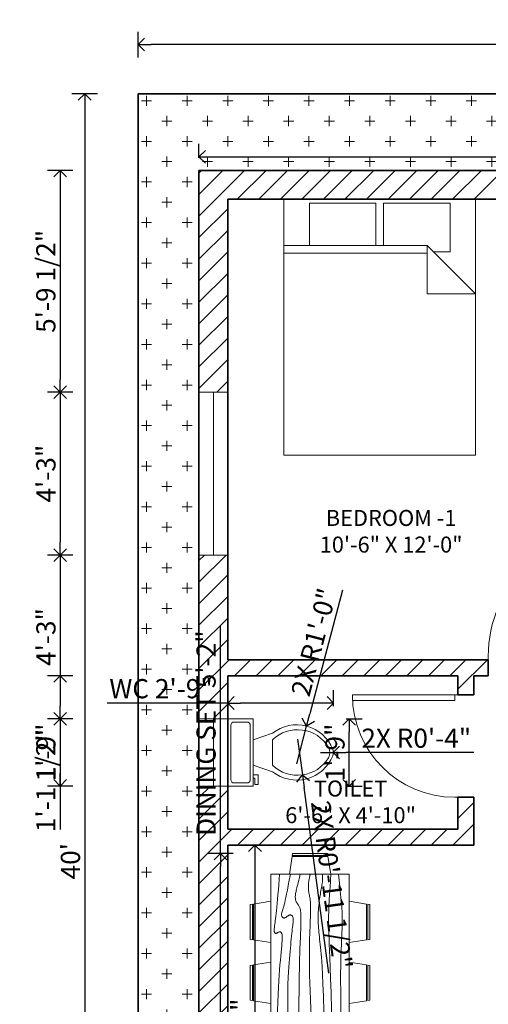
# Model space of a CAD drawing. Units: inches. Extents: x 686 to 1065, y 83 to 664.
# Tile 3 of 5: x 686 to 833, y 308 to 616. Entities that reach past the tile are written whole.
import ezdxf

# ---------------------------------------------------------------- set-up
doc = ezdxf.new("R2010")
doc.units = ezdxf.units.IN
for name, color, linetype, lineweight in [('A-ANNO-DIMS', 2, 'Continuous', 18), ('A-AREA-IDEN', 7, 'Continuous', 20), ('A-DOOR', 4, 'Continuous', 20), ('A-FLOR-FIXT', 9, 'Continuous', 18), ('A-FURN', 8, 'Continuous', 18), ('A-GLAZ', 172, 'Continuous', 18), ('A-WALL', 7, 'Continuous', 35), ('A-WALL-PATT', 253, 'Continuous', 13), ('C-PROP', 7, 'Continuous', 35), ('L-SITE-PATT', 94, 'Continuous', 13)]:
    doc.layers.add(name, color=color, linetype=linetype, lineweight=lineweight)
doc.styles.get("Standard").update_dxf_attribs({"font": 'arial.ttf'})
doc.dimstyles.new('ISO-25', dxfattribs={"dimtxt": 6, "dimasz": 4, "dimexe": 4, "dimexo": 4, "dimtad": 1, "dimdec": 1, "dimlunit": 3, "dimtxsty": 'Standard', "dimblk": 'OPEN90', "dimcen": 2.5, "dimadec": 0, "dimazin": 0, "dimtfac": 1, "dimtdec": 1, "dimtmove": 0, "dimatfit": 3, "dimfxl": 4, "dimfxlon": 1, "dimarcsym": 0})

# ---------------------------------------------------------------- blocks, each defined once
blk = doc.blocks.new('_Open90')
at = {"color": 0, "linetype": 'ByBlock', "lineweight": -2}
for p, q in [((0, 0), (-1, 0)), ((-0.5, 0.5), (0, 0)), ((0, 0), (-0.5, -0.5))]:
    blk.add_line(p, q, dxfattribs=at)
blk = doc.blocks.new('*D11')
at = {"layer": 'A-ANNO-DIMS', "color": 0, "lineweight": -2, "transparency": 16777216}
for p, q in [((742.37, 572.73), (742.37, 577.04)), ((1011.37, 572.73), (1011.37, 577.04)), ((746.37, 573.04), (1007.37, 573.04))]:
    blk.add_line(p, q, dxfattribs=at)
at = {"layer": 'Defpoints', "color": 0, "transparency": 16777216}
for p in [(1011.37, 573.04), (742.37, 568.73), (1011.37, 568.73)]:
    blk.add_point(p, dxfattribs=at)
at = {"layer": 'A-ANNO-DIMS', "color": 0, "lineweight": -2, "transparency": 16777216, "xscale": 4, "yscale": 4, "zscale": 4, "rotation": 180}
blk.add_blockref('_Open90', (742.37, 573.04), dxfattribs=at)
at = {"layer": 'A-ANNO-DIMS', "color": 0, "lineweight": -2, "transparency": 16777216, "xscale": 4, "yscale": 4, "zscale": 4}
blk.add_blockref('_Open90', (1011.37, 573.04), dxfattribs=at)
at = {"layer": 'A-ANNO-DIMS', "color": 0, "transparency": 16777216, "insert": (876.87, 576.73), "char_height": 6, "attachment_point": 5}
blk.add_mtext('22\'-5"', dxfattribs=at)
blk = doc.blocks.new('*D13')
at = {"layer": 'A-ANNO-DIMS', "color": 0, "lineweight": -2, "transparency": 16777216}
for p, q in [((755.89, 357.73), (763.89, 357.73)), ((759.89, 353.73), (759.89, 247.73)), ((755.89, 243.73), (763.89, 243.73))]:
    blk.add_line(p, q, dxfattribs=at)
at = {"layer": 'Defpoints', "color": 0, "transparency": 16777216}
for p in [(751.37, 357.73), (751.37, 243.73), (759.89, 243.73)]:
    blk.add_point(p, dxfattribs=at)
at = {"layer": 'A-ANNO-DIMS', "color": 0, "lineweight": -2, "transparency": 16777216, "xscale": 4, "yscale": 4, "zscale": 4}
for p, rotation in [((759.89, 357.73), 90), ((759.89, 243.73), 270)]:
    blk.add_blockref('_Open90', p, dxfattribs=dict(at, rotation=rotation))
at = {"layer": 'A-ANNO-DIMS', "color": 0, "transparency": 16777216, "insert": (756.2, 300.73), "char_height": 6, "attachment_point": 5, "rotation": 90}
blk.add_mtext('8\'-1"', dxfattribs=at)
blk = doc.blocks.new('Toilet - top')
for p, q in [((9.5, -6), (9.5, -2)), ((-10, -8.5), (-8, -8.5)), ((-10, -9.5), (-10, -8.5)), ((-8, -8.5), (-8, -8)), ((-7, -8), (-7, -9.5)), ((-4, -8), (-6, -14)), ((4, -8), (6, -14)), ((-7, -9.5), (-10, -9.5)), ((4, -14), (-4, -14))]:
    blk.add_line(p, q)
blk.add_lwpolyline([(10.5, -8), (10.5, 0), (-10.5, 0), (-10.5, -8)], close=True)
for points in [[(-9.5, -2), (-9.5, -6)], [(8.5, -1), (-8.5, -1)], [(-8.5, -7), (8.5, -7)]]:
    blk.add_lwpolyline(points)
for centre, radius, start, end in [((-8.62, -1.88), 0.884, 81.8699, 188.1301), ((8.62, -1.88), 0.884, 351.8699, 98.1301), ((-8.62, -6.12), 0.884, 171.8699, 278.1301), ((8.62, -6.12), 0.884, 261.8699, 8.1301), ((3.52, -21.58), 12.17, 141.4691, 247.9714), ((4.2, -21.82), 11.33, 136.3677, 238.9468), ((-3.52, -21.58), 12.17, 292.0284, 38.5307), ((-4.2, -21.82), 11.33, 301.053, 43.6321), ((0, -27.88), 4, 245.7318, 294.2682), ((0, -29), 4, 254.8605, 285.1395)]:
    blk.add_arc(centre, radius, start, end)
blk = doc.blocks.new('Bed - Queen')
for p, q in [((0, -80.00003), (0, 0)), ((0, 0), (59.99999, 0)), ((59.99999, 0), (59.99999, -80.00003)), ((7.99999, -1.2), (28.79998, -1.2)), ((7.99999, -14.4), (7.99999, -1.2)), ((28.79998, -1.2), (28.79998, -14.4)), ((31.19999, -1.2), (51.99999, -1.2)), ((31.19999, -14.4), (31.19999, -1.2)), ((51.99999, -1.2), (51.99999, -16.4)), ((0, -14.4), (44.8, -14.4)), ((59.99999, -29.6), (44.8, -14.4)), ((44.8, -14.4), (44.8, -29.6)), ((44.8, -16.8), (0, -16.8)), ((51.99999, -16.4), (46.79936, -16.4)), ((44.8, -29.6), (59.99999, -29.6)), ((59.99999, -80.00003), (0, -80.00003))]:
    blk.add_line(p, q)
blk = doc.blocks.new('Dining Set - 36 x 72 in.')
for p, q in [((-22, 27.5), (-22.1562, 26.50042)), ((-22, 27.5), (-6, 27.5)), ((-5.8437, 26.49966), (-6, 27.5)), ((6, 27.5), (5.8438, 26.50042)), ((6, 27.5), (22, 27.5)), ((22.1563, 26.49966), (22, 27.5)), ((-22.2343, 26.00059), (-23.4847, 17.99762)), ((-22.2304, 26), (-5.7608, 26)), ((-5.8416, 26.5), (-22.1534, 26.5)), ((-4.5152, 17.99762), (-5.7655, 25.99926)), ((5.7657, 26.00059), (4.5153, 17.99762)), ((5.7696, 26), (22.2392, 26)), ((22.1584, 26.5), (5.8466, 26.5)), ((23.4848, 17.99762), (22.2345, 25.99926)), ((36, 18), (-36, 18)), ((-36, 18), (-36, -18)), ((36, -18), (36, 18)), ((-44.0006, 8.23428), (-35.9976, 9.48474)), ((44.0006, 8.23428), (35.9976, 9.48474)), ((-45.5, 8), (-44.5004, 8.15617)), ((-45.5, 8), (-45.5, -8)), ((-44.5, -8.15843), (-44.5, 8.15338)), ((-44, 8.23041), (-44, -8.23915)), ((44, 8.23041), (44, -8.23915)), ((44.5, -8.15843), (44.5, 8.15338)), ((45.5, 8), (44.5005, 8.15617)), ((45.5, 8), (45.5, -8)), ((-44.4997, -8.15631), (-45.5, -8)), ((-35.9976, -9.48476), (-43.9993, -8.2345)), ((35.9976, -9.48476), (43.9993, -8.2345)), ((44.4997, -8.15631), (45.5, -8)), ((-36, -18), (36, -18)), ((-22.2343, -26.0006), (-23.4847, -17.99762)), ((-4.5152, -17.99762), (-5.7655, -25.99928)), ((5.7657, -26.0006), (4.5153, -17.99762)), ((23.4848, -17.99762), (22.2345, -25.99928)), ((-22.2304, -26), (-5.7608, -26)), ((-22, -27.5), (-22.1562, -26.50044)), ((-5.8416, -26.5), (-22.1534, -26.5)), ((-5.8437, -26.49967), (-6, -27.5)), ((5.7696, -26), (22.2392, -26)), ((6, -27.5), (5.8438, -26.50044)), ((22.1584, -26.5), (5.8466, -26.5)), ((22.1563, -26.49967), (22, -27.5)), ((-22, -27.5), (-6, -27.5)), ((6, -27.5), (22, -27.5))]:
    blk.add_line(p, q)
for points in [[(-36, 15), (-31.1772, 14.97754), (-26.8079, 14.91406), (-22.8538, 14.81543), (-19.276, 14.6875), (-16.0362, 14.53613), (-13.0957, 14.36718), (-10.4159, 14.18652), (-7.9583, 14), (-5.6904, 13.81315), (-3.6035, 13.63021), (-1.6954, 13.45508), (0.0365, 13.29166), (1.5945, 13.14388), (2.9811, 13.01562), (4.1988, 12.9108), (5.25, 12.83333), (6.1393, 12.78613), (6.8802, 12.76823), (7.4883, 12.77767), (7.9792, 12.8125), (8.3685, 12.87077), (8.6719, 12.95052), (8.9049, 13.0498), (9.0833, 13.16666), (9.2205, 13.29899), (9.3216, 13.44401), (9.3895, 13.59879), (9.4271, 13.76041), (9.4373, 13.92594), (9.4232, 14.09245), (9.3875, 14.257), (9.3333, 14.41666), (9.2638, 14.56917), (9.1836, 14.71484), (9.0975, 14.85465), (9.0104, 14.98958), (8.9272, 15.1206), (8.8529, 15.2487), (8.7922, 15.37483), (8.75, 15.5), (8.7305, 15.62467), (8.7344, 15.74739), (8.7617, 15.86621), (8.8125, 15.97916), (8.8867, 16.08431), (8.9844, 16.17968), (9.1055, 16.26334), (9.25, 16.33333), (9.4189, 16.38802), (9.6172, 16.42708), (9.8506, 16.45052), (10.125, 16.45833), (10.4463, 16.45052), (10.8203, 16.42708), (11.2529, 16.38802), (11.75, 16.33333), (12.3184, 16.26318), (12.9694, 16.17838), (13.7151, 16.07991), (14.5677, 15.96875), (15.5395, 15.84586), (16.6426, 15.71224), (17.8893, 15.56884), (19.2917, 15.41666), (20.859, 15.25667), (22.5879, 15.08984), (24.4721, 14.91715), (26.5052, 14.73958), (28.6809, 14.5581), (30.9929, 14.3737), (33.4347, 14.18733), (36, 14)], [(-36, 10), (-28.9766, 10.14274), (-23.1725, 10.20442), (-18.4241, 10.19775), (-14.5677, 10.13541), (-11.4399, 10.03011), (-8.877, 9.89453), (-6.7154, 9.74137), (-4.7917, 9.58333), (-2.9698, 9.43082), (-1.2246, 9.28515), (0.4415, 9.14534), (2.026, 9.01041), (3.5266, 8.87939), (4.9408, 8.7513), (6.266, 8.62516), (7.5, 8.5), (8.6411, 8.37549), (9.6914, 8.2539), (10.6538, 8.13818), (11.5312, 8.03125), (12.3267, 7.93603), (13.043, 7.85547), (13.6831, 7.79248), (14.25, 7.75), (14.7471, 7.7303), (15.1797, 7.73307), (15.5537, 7.75732), (15.875, 7.80208), (16.1494, 7.86637), (16.3828, 7.94922), (16.5811, 8.04964), (16.75, 8.16666), (16.8944, 8.29915), (17.0143, 8.44531), (17.1089, 8.60319), (17.1771, 8.77083), (17.218, 8.94629), (17.2305, 9.1276), (17.2137, 9.31282), (17.1667, 9.5), (17.0895, 9.6875), (16.987, 9.875), (16.8649, 10.0625), (16.7292, 10.25), (16.5856, 10.4375), (16.4401, 10.625), (16.2985, 10.8125), (16.1667, 11), (16.05, 11.18733), (15.9518, 11.3737), (15.8752, 11.5581), (15.8229, 11.73958), (15.798, 11.91715), (15.8034, 12.08984), (15.842, 12.25667), (15.9167, 12.41666), (16.0295, 12.56836), (16.1784, 12.70833), (16.3605, 12.83268), (16.5729, 12.9375), (16.8127, 13.01888), (17.0768, 13.07291), (17.3625, 13.0957), (17.6667, 13.08333), (17.9894, 13.03312), (18.3418, 12.94726), (18.7382, 12.82918), (19.1927, 12.68229), (19.7195, 12.51001), (20.3327, 12.31575), (21.0465, 12.10294), (21.875, 11.875), (22.8357, 11.63354), (23.959, 11.37304), (25.2786, 11.08618), (26.8282, 10.76562), (28.6414, 10.40405), (30.752, 9.99414), (33.1936, 9.52856), (36, 9)], [(-36, 5.5), (-30.7157, 5.3348), (-26.069, 5.20963), (-21.9946, 5.11767), (-18.4271, 5.05208), (-15.3009, 5.00602), (-12.5508, 4.97265), (-10.1112, 4.94515), (-7.9167, 4.91666), (-5.909, 4.88167), (-4.0586, 4.83984), (-2.3429, 4.79215), (-0.7396, 4.73958), (0.7739, 4.6831), (2.22, 4.6237), (3.6213, 4.56233), (5, 4.5), (6.373, 4.43782), (7.7344, 4.3776), (9.0723, 4.32129), (10.375, 4.27083), (11.6309, 4.22819), (12.8281, 4.19531), (13.9551, 4.17415), (15, 4.16666), (15.954, 4.17448), (16.819, 4.19791), (17.6001, 4.23698), (18.3021, 4.29166), (18.9299, 4.36198), (19.4883, 4.44791), (19.9823, 4.54948), (20.4167, 4.66666), (20.7969, 4.79899), (21.1302, 4.94401), (21.4245, 5.09879), (21.6875, 5.26041), (21.9271, 5.42594), (22.1511, 5.59245), (22.3672, 5.757), (22.5834, 5.91666), (22.8065, 6.06868), (23.0404, 6.21093), (23.2879, 6.34147), (23.5521, 6.45833), (23.8358, 6.55957), (24.142, 6.64323), (24.4735, 6.70735), (24.8334, 6.75), (25.2235, 6.76969), (25.642, 6.76692), (26.0858, 6.74267), (26.5521, 6.69791), (27.0379, 6.63362), (27.5404, 6.55078), (28.0565, 6.45036), (28.5834, 6.33333), (29.1242, 6.19987), (29.7071, 6.04687), (30.3661, 5.87044), (31.1354, 5.66666), (32.0493, 5.43164), (33.142, 5.16146), (34.4475, 4.85221), (36, 4.5)], [(-36, -1), (-30.7915, -0.6591), (-26.0195, -0.38216), (-21.6519, -0.16284), (-17.6563, 0.00521), (-14.0005, 0.12833), (-10.6523, 0.21289), (-7.5796, 0.26522), (-4.75, 0.29166), (-2.134, 0.29793), (0.2878, 0.28711), (2.5317, 0.26163), (4.6146, 0.22396), (6.5529, 0.17651), (8.3633, 0.12174), (10.0623, 0.06209), (11.6667, 0), (13.1899, -0.06201), (14.6341, -0.1211), (15.9982, -0.17432), (17.2813, -0.21875), (18.4823, -0.25147), (19.6003, -0.26953), (20.6343, -0.27002), (21.5834, -0.25), (22.4481, -0.20768), (23.2357, -0.14584), (23.9549, -0.06836), (24.6146, 0.02083), (25.2235, 0.11784), (25.7904, 0.21875), (26.3241, 0.31966), (26.8334, 0.41666), (27.3265, 0.50618), (27.8099, 0.58593), (28.2894, 0.65397), (28.7709, 0.70833), (29.2601, 0.74707), (29.763, 0.76823), (30.2855, 0.76985), (30.8334, 0.75), (31.4088, 0.70784), (31.9994, 0.64713), (32.589, 0.57275), (33.1615, 0.48958), (33.7008, 0.4025), (34.1908, 0.3164), (34.6153, 0.23616), (34.9584, 0.16666), (35.2099, 0.11165), (35.3848, 0.07031), (35.504, 0.04069), (35.5886, 0.02083), (35.6594, 0.00879), (35.7377, 0.0026), (35.8442, 0.00032), (36, 0)], [(-36, -6.5), (-27.1843, -6.31267), (-20.084, -6.1263), (-14.469, -5.9419), (-10.1094, -5.76042), (-6.7752, -5.58285), (-4.2363, -5.41016), (-2.2629, -5.24333), (-0.625, -5.08334), (0.8708, -4.93099), (2.2715, -4.78646), (3.5872, -4.64974), (4.8281, -4.52084), (6.0046, -4.39974), (7.127, -4.28646), (8.2053, -4.18099), (9.25, -4.08334), (10.2705, -3.99382), (11.2734, -3.91407), (12.2647, -3.84603), (13.25, -3.79167), (14.2354, -3.75293), (15.2266, -3.73177), (16.2295, -3.73015), (17.25, -3.75), (18.2912, -3.79248), (19.3451, -3.85547), (20.4009, -3.93604), (21.4479, -4.03125), (22.4754, -4.13819), (23.4727, -4.25391), (24.4289, -4.37549), (25.3334, -4.5), (26.1785, -4.62492), (26.9694, -4.74935), (27.7145, -4.87281), (28.4219, -4.99479), (29.1, -5.11483), (29.7572, -5.23242), (30.4016, -5.34709), (31.0417, -5.45834), (31.6837, -5.56437), (32.3262, -5.65821), (32.9658, -5.73153), (33.599, -5.77604), (34.2224, -5.78345), (34.8327, -5.74545), (35.4264, -5.65373), (36, -5.5)], [(-36, -10), (-26.4022, -9.81299), (-18.4675, -9.62891), (-11.9839, -9.45069), (-6.7396, -9.28125), (-2.5226, -9.12354), (0.8789, -8.98047), (3.6769, -8.85498), (6.0833, -8.75), (8.2767, -8.66765), (10.3021, -8.60677), (12.1712, -8.56543), (13.8958, -8.54167), (15.4876, -8.53353), (16.9583, -8.53907), (18.3197, -8.55632), (19.5834, -8.58334), (20.7616, -8.61841), (21.8685, -8.66081), (22.9188, -8.71004), (23.9271, -8.76563), (24.9081, -8.82707), (25.8763, -8.89388), (26.8465, -8.96558), (27.8334, -9.04167), (28.8474, -9.12118), (29.8828, -9.20117), (30.93, -9.27824), (31.9792, -9.34896), (33.0205, -9.40991), (34.0443, -9.45768), (35.0407, -9.48885), (36, -9.5)], [(-36, -14.5), (-30.0881, -14.33513), (-25.0332, -14.21224), (-20.7312, -14.12647), (-17.0781, -14.07292), (-13.97, -14.04671), (-11.3027, -14.04297), (-8.9724, -14.05681), (-6.875, -14.08334), (-4.9224, -14.11833), (-3.0905, -14.16016), (-1.3709, -14.20785), (0.2448, -14.26042), (1.7647, -14.3169), (3.1973, -14.3763), (4.5507, -14.43767), (5.8333, -14.5), (7.0554, -14.5621), (8.235, -14.62175), (9.3922, -14.67652), (10.5469, -14.72396), (11.7192, -14.76164), (12.929, -14.78711), (14.1965, -14.79794), (15.5417, -14.79167), (16.9933, -14.76424), (18.6152, -14.70508), (20.4804, -14.60197), (22.6615, -14.44271), (25.2312, -14.21509), (28.2624, -13.9069), (31.8277, -13.50594), (36, -13)]]:
    blk.add_lwpolyline(points)
blk = doc.blocks.new('*D17')
at = {"layer": 'A-ANNO-DIMS', "color": 0, "lineweight": -2, "transparency": 16777216}
for p, q in [((723.37, 604.13), (723.37, 612.13)), ((1023.37, 604.13), (1023.37, 612.13)), ((1019.37, 608.13), (727.37, 608.13))]:
    blk.add_line(p, q, dxfattribs=at)
at = {"layer": 'Defpoints', "color": 0, "transparency": 16777216}
for p in [(723.37, 608.13), (723.37, 592.73), (1023.37, 592.73)]:
    blk.add_point(p, dxfattribs=at)
at = {"layer": 'A-ANNO-DIMS', "color": 0, "lineweight": -2, "transparency": 16777216, "xscale": 4, "yscale": 4, "zscale": 4, "rotation": 180}
blk.add_blockref('_Open90', (723.37, 608.13), dxfattribs=at)
at = {"layer": 'A-ANNO-DIMS', "color": 0, "lineweight": -2, "transparency": 16777216, "xscale": 4, "yscale": 4, "zscale": 4}
blk.add_blockref('_Open90', (1023.37, 608.13), dxfattribs=at)
at = {"layer": 'A-ANNO-DIMS', "color": 0, "transparency": 16777216, "insert": (873.37, 611.82), "char_height": 6, "attachment_point": 5}
blk.add_mtext("25'", dxfattribs=at)
blk = doc.blocks.new('*D18')
at = {"layer": 'A-ANNO-DIMS', "color": 0, "lineweight": -2, "transparency": 16777216}
for p, q in [((710.63, 592.73), (702.63, 592.73)), ((706.63, 588.73), (706.63, 116.73)), ((710.63, 112.73), (702.63, 112.73))]:
    blk.add_line(p, q, dxfattribs=at)
at = {"layer": 'Defpoints', "color": 0, "transparency": 16777216}
for p in [(723.37, 592.73), (706.63, 112.73), (723.37, 112.73)]:
    blk.add_point(p, dxfattribs=at)
at = {"layer": 'A-ANNO-DIMS', "color": 0, "lineweight": -2, "transparency": 16777216, "xscale": 4, "yscale": 4, "zscale": 4}
for p, rotation in [((706.63, 592.73), 90), ((706.63, 112.73), 270)]:
    blk.add_blockref('_Open90', p, dxfattribs=dict(at, rotation=rotation))
at = {"layer": 'A-ANNO-DIMS', "color": 0, "transparency": 16777216, "insert": (702.94, 352.73), "char_height": 6, "attachment_point": 5, "rotation": 90}
blk.add_mtext("40'", dxfattribs=at)
blk = doc.blocks.new('*U23')
for p, q in [((0, 0), (0, -6)), ((-40, 0), (-40, -6))]:
    blk.add_line(p, q)
blk.add_lwpolyline([(0, 0), (0, 40), (-1.75, 40), (-1.75, 0)], close=True)
blk.add_arc((0, 0), 40, 90, 180)
blk = doc.blocks.new('*U22')
for p, q in [((0, 0), (0, -6)), ((-32, 0), (-32, -6))]:
    blk.add_line(p, q)
blk.add_lwpolyline([(0, 0), (0, 32), (-1.75, 32), (-1.75, 0)], close=True)
blk.add_arc((0, 0), 32, 90, 180)
blk = doc.blocks.new('*D30')
at = {"layer": 'A-ANNO-DIMS', "color": 0, "lineweight": -2, "transparency": 16777216}
for p, q in [((751.37, 401.23), (751.37, 406.19)), ((784.42, 401.23), (784.42, 406.19)), ((751.37, 402.19), (713.63, 402.19)), ((780.42, 402.19), (755.37, 402.19))]:
    blk.add_line(p, q, dxfattribs=at)
at = {"layer": 'Defpoints', "color": 0, "transparency": 16777216}
for p in [(751.37, 402.19), (751.37, 397.23), (784.42, 397.23)]:
    blk.add_point(p, dxfattribs=at)
at = {"layer": 'A-ANNO-DIMS', "color": 0, "lineweight": -2, "transparency": 16777216, "xscale": 4, "yscale": 4, "zscale": 4, "rotation": 180}
blk.add_blockref('_Open90', (751.37, 402.19), dxfattribs=at)
at = {"layer": 'A-ANNO-DIMS', "color": 0, "lineweight": -2, "transparency": 16777216, "xscale": 4, "yscale": 4, "zscale": 4}
blk.add_blockref('_Open90', (784.42, 402.19), dxfattribs=at)
at = {"layer": 'A-ANNO-DIMS', "color": 0, "transparency": 16777216, "insert": (730.5, 405.91), "char_height": 6, "attachment_point": 5}
blk.add_mtext('WC 2\'-9"', dxfattribs=at)
blk = doc.blocks.new('*D31')
at = {"layer": 'A-ANNO-DIMS', "color": 0, "lineweight": -2, "transparency": 16777216}
for p, q in [((788.42, 397.23), (793.37, 397.23)), ((789.37, 380.23), (789.37, 393.23)), ((788.42, 376.23), (793.37, 376.23))]:
    blk.add_line(p, q, dxfattribs=at)
at = {"layer": 'Defpoints', "color": 0, "transparency": 16777216}
for p in [(784.42, 397.23), (789.37, 397.23), (784.42, 376.23)]:
    blk.add_point(p, dxfattribs=at)
at = {"layer": 'A-ANNO-DIMS', "color": 0, "lineweight": -2, "transparency": 16777216, "xscale": 4, "yscale": 4, "zscale": 4}
for p, rotation in [((789.37, 397.23), 90), ((789.37, 376.23), 270)]:
    blk.add_blockref('_Open90', p, dxfattribs=dict(at, rotation=rotation))
at = {"layer": 'A-ANNO-DIMS', "color": 0, "transparency": 16777216, "insert": (785.69, 386.73), "char_height": 6, "attachment_point": 5, "rotation": 90}
blk.add_mtext('1\'-9"', dxfattribs=at)
blk = doc.blocks.new('*D34')
at = {"layer": 'A-ANNO-DIMS', "color": 0, "lineweight": -2, "transparency": 16777216}
for p, q in [((749.09, 355.19), (749.09, 426.38)), ((753.09, 355.19), (745.09, 355.19)), ((749.09, 297.22), (749.09, 351.19)), ((753.09, 293.22), (745.09, 293.22))]:
    blk.add_line(p, q, dxfattribs=at)
at = {"layer": 'Defpoints', "color": 0, "transparency": 16777216}
for p in [(749.09, 355.19), (758.38, 355.19), (758.38, 293.22)]:
    blk.add_point(p, dxfattribs=at)
at = {"layer": 'A-ANNO-DIMS', "color": 0, "lineweight": -2, "transparency": 16777216, "xscale": 4, "yscale": 4, "zscale": 4}
for p, rotation in [((749.09, 355.19), 90), ((749.09, 293.22), 270)]:
    blk.add_blockref('_Open90', p, dxfattribs=dict(at, rotation=rotation))
at = {"layer": 'A-ANNO-DIMS', "color": 0, "transparency": 16777216, "insert": (745.36, 392.78), "char_height": 6, "attachment_point": 5, "rotation": 90}
blk.add_mtext('DINING SET 5\'-2"', dxfattribs=at)
blk = doc.blocks.new('*D42')
at = {"layer": 'A-ANNO-DIMS', "color": 0, "lineweight": -2, "transparency": 16777216}
for p, q in [((702.96, 568.73), (694.96, 568.73)), ((698.96, 564.73), (698.96, 503.41)), ((702.96, 499.41), (694.96, 499.41))]:
    blk.add_line(p, q, dxfattribs=at)
at = {"layer": 'Defpoints', "color": 0, "transparency": 16777216}
for p in [(742.37, 568.73), (698.96, 499.41), (742.37, 499.41)]:
    blk.add_point(p, dxfattribs=at)
at = {"layer": 'A-ANNO-DIMS', "color": 0, "lineweight": -2, "transparency": 16777216, "xscale": 4, "yscale": 4, "zscale": 4}
for p, rotation in [((698.96, 568.73), 90), ((698.96, 499.41), 270)]:
    blk.add_blockref('_Open90', p, dxfattribs=dict(at, rotation=rotation))
at = {"layer": 'A-ANNO-DIMS', "color": 0, "transparency": 16777216, "insert": (695.23, 534.07), "char_height": 6, "attachment_point": 5, "rotation": 90}
blk.add_mtext('5\'-9 1/2"', dxfattribs=at)
blk = doc.blocks.new('*D43')
at = {"layer": 'A-ANNO-DIMS', "color": 0, "lineweight": -2, "transparency": 16777216}
for p, q in [((702.96, 499.41), (694.96, 499.41)), ((698.96, 495.41), (698.96, 452.47)), ((702.96, 448.47), (694.96, 448.47))]:
    blk.add_line(p, q, dxfattribs=at)
at = {"layer": 'Defpoints', "color": 0, "transparency": 16777216}
for p in [(742.37, 499.41), (698.96, 448.47), (742.37, 448.47)]:
    blk.add_point(p, dxfattribs=at)
at = {"layer": 'A-ANNO-DIMS', "color": 0, "lineweight": -2, "transparency": 16777216, "xscale": 4, "yscale": 4, "zscale": 4}
for p, rotation in [((698.96, 499.41), 90), ((698.96, 448.47), 270)]:
    blk.add_blockref('_Open90', p, dxfattribs=dict(at, rotation=rotation))
at = {"layer": 'A-ANNO-DIMS', "color": 0, "transparency": 16777216, "insert": (695.27, 473.94), "char_height": 6, "attachment_point": 5, "rotation": 90}
blk.add_mtext('4\'-3"', dxfattribs=at)
blk = doc.blocks.new('*D44')
at = {"layer": 'A-ANNO-DIMS', "color": 0, "lineweight": -2, "transparency": 16777216}
for p, q in [((702.96, 448.47), (694.96, 448.47)), ((698.96, 444.47), (698.96, 401.23)), ((702.96, 397.23), (694.96, 397.23))]:
    blk.add_line(p, q, dxfattribs=at)
at = {"layer": 'Defpoints', "color": 0, "transparency": 16777216}
for p in [(742.37, 448.47), (698.96, 397.23), (742.37, 397.23)]:
    blk.add_point(p, dxfattribs=at)
at = {"layer": 'A-ANNO-DIMS', "color": 0, "lineweight": -2, "transparency": 16777216, "xscale": 4, "yscale": 4, "zscale": 4}
for p, rotation in [((698.96, 448.47), 90), ((698.96, 397.23), 270)]:
    blk.add_blockref('_Open90', p, dxfattribs=dict(at, rotation=rotation))
at = {"layer": 'A-ANNO-DIMS', "color": 0, "transparency": 16777216, "insert": (695.27, 422.85), "char_height": 6, "attachment_point": 5, "rotation": 90}
blk.add_mtext('4\'-3"', dxfattribs=at)
blk = doc.blocks.new('*D45')
at = {"layer": 'A-ANNO-DIMS', "color": 0, "lineweight": -2, "transparency": 16777216}
for p, q in [((702.96, 397.23), (694.96, 397.23)), ((698.96, 393.23), (698.96, 380.23)), ((702.96, 376.23), (694.96, 376.23))]:
    blk.add_line(p, q, dxfattribs=at)
at = {"layer": 'Defpoints', "color": 0, "transparency": 16777216}
for p in [(742.37, 397.23), (698.96, 376.23), (742.37, 376.23)]:
    blk.add_point(p, dxfattribs=at)
at = {"layer": 'A-ANNO-DIMS', "color": 0, "lineweight": -2, "transparency": 16777216, "xscale": 4, "yscale": 4, "zscale": 4}
for p, rotation in [((698.96, 397.23), 90), ((698.96, 376.23), 270)]:
    blk.add_blockref('_Open90', p, dxfattribs=dict(at, rotation=rotation))
at = {"layer": 'A-ANNO-DIMS', "color": 0, "transparency": 16777216, "insert": (695.27, 386.73), "char_height": 6, "attachment_point": 5, "rotation": 90}
blk.add_mtext('1\'-9"', dxfattribs=at)
blk = doc.blocks.new('*D57')
at = {"layer": 'A-ANNO-DIMS', "color": 0, "lineweight": -2, "transparency": 16777216}
for p, q in [((1043.78, 404.73), (1051.78, 404.73)), ((1047.78, 400.73), (1047.78, 376.73)), ((1043.78, 372.73), (1051.78, 372.73))]:
    blk.add_line(p, q, dxfattribs=at)
at = {"layer": 'Defpoints', "color": 0, "transparency": 16777216}
for p in [(828.37, 404.73), (828.37, 372.73), (1047.78, 372.73)]:
    blk.add_point(p, dxfattribs=at)
at = {"layer": 'A-ANNO-DIMS', "color": 0, "lineweight": -2, "transparency": 16777216, "xscale": 4, "yscale": 4, "zscale": 4}
for p, rotation in [((1047.78, 404.73), 90), ((1047.78, 372.73), 270)]:
    blk.add_blockref('_Open90', p, dxfattribs=dict(at, rotation=rotation))
at = {"layer": 'A-ANNO-DIMS', "color": 0, "transparency": 16777216, "insert": (1044.09, 388.73), "char_height": 6, "attachment_point": 5, "rotation": 90}
blk.add_mtext('2\'-8"', dxfattribs=at)
blk = doc.blocks.new('*D61')
at = {"layer": 'A-ANNO-DIMS', "color": 0, "lineweight": -2, "transparency": 16777216}
for p, q in [((1043.78, 372.73), (1051.78, 372.73)), ((1047.78, 368.73), (1047.78, 366.73)), ((1043.78, 362.73), (1051.78, 362.73)), ((1047.78, 362.73), (1047.78, 336.87))]:
    blk.add_line(p, q, dxfattribs=at)
at = {"layer": 'Defpoints', "color": 0, "transparency": 16777216}
for p in [(823.37, 372.73), (823.37, 362.73), (1047.78, 362.73)]:
    blk.add_point(p, dxfattribs=at)
at = {"layer": 'A-ANNO-DIMS', "color": 0, "lineweight": -2, "transparency": 16777216, "xscale": 4, "yscale": 4, "zscale": 4}
for p, rotation in [((1047.78, 372.73), 90), ((1047.78, 362.73), 270)]:
    blk.add_blockref('_Open90', p, dxfattribs=dict(at, rotation=rotation))
at = {"layer": 'A-ANNO-DIMS', "color": 0, "transparency": 16777216, "insert": (1044.09, 347.8), "char_height": 6, "attachment_point": 5, "rotation": 90}
blk.add_mtext('0\'-10"', dxfattribs=at)
blk = doc.blocks.new('*D62')
at = {"layer": 'A-ANNO-DIMS', "color": 0, "lineweight": -2, "transparency": 16777216}
for p, q in [((742.37, 92.32), (742.37, 84.32)), ((751.37, 92.32), (751.37, 84.32)), ((738.37, 88.32), (734.37, 88.32)), ((742.37, 88.32), (751.37, 88.32)), ((755.37, 88.32), (776.57, 88.32))]:
    blk.add_line(p, q, dxfattribs=at)
at = {"layer": 'Defpoints', "color": 0, "transparency": 16777216}
for p in [(742.37, 376.23), (751.37, 376.23), (751.37, 88.32)]:
    blk.add_point(p, dxfattribs=at)
at = {"layer": 'A-ANNO-DIMS', "color": 0, "lineweight": -2, "transparency": 16777216, "xscale": 4, "yscale": 4, "zscale": 4}
blk.add_blockref('_Open90', (742.37, 88.32), dxfattribs=at)
at = {"layer": 'A-ANNO-DIMS', "color": 0, "lineweight": -2, "transparency": 16777216, "xscale": 4, "yscale": 4, "zscale": 4, "rotation": 180}
blk.add_blockref('_Open90', (751.37, 88.32), dxfattribs=at)
at = {"layer": 'A-ANNO-DIMS', "color": 0, "transparency": 16777216, "insert": (767.97, 92.01), "char_height": 6, "attachment_point": 5}
blk.add_mtext('0\'-9"', dxfattribs=at)
blk = doc.blocks.new('*D63')
at = {"layer": 'A-ANNO-DIMS', "color": 0, "lineweight": -2, "transparency": 16777216}
for p, q in [((823.37, 92.32), (823.37, 84.32)), ((828.37, 92.32), (828.37, 84.32)), ((819.37, 88.32), (815.37, 88.32)), ((823.37, 88.32), (828.37, 88.32)), ((832.37, 88.32), (853.57, 88.32))]:
    blk.add_line(p, q, dxfattribs=at)
at = {"layer": 'Defpoints', "color": 0, "transparency": 16777216}
for p in [(823.37, 362.73), (828.37, 357.73), (828.37, 88.32)]:
    blk.add_point(p, dxfattribs=at)
at = {"layer": 'A-ANNO-DIMS', "color": 0, "lineweight": -2, "transparency": 16777216, "xscale": 4, "yscale": 4, "zscale": 4}
blk.add_blockref('_Open90', (823.37, 88.32), dxfattribs=at)
at = {"layer": 'A-ANNO-DIMS', "color": 0, "lineweight": -2, "transparency": 16777216, "xscale": 4, "yscale": 4, "zscale": 4, "rotation": 180}
blk.add_blockref('_Open90', (828.37, 88.32), dxfattribs=at)
at = {"layer": 'A-ANNO-DIMS', "color": 0, "transparency": 16777216, "insert": (844.97, 92.01), "char_height": 6, "attachment_point": 5}
blk.add_mtext('0\'-5"', dxfattribs=at)
blk = doc.blocks.new('*D73')
at = {"layer": 'A-ANNO-DIMS', "color": 0, "lineweight": -2, "transparency": 16777216}
for p, q in [((702.96, 410.73), (694.96, 410.73)), ((698.96, 406.73), (698.96, 401.23)), ((702.96, 397.23), (694.96, 397.23)), ((698.96, 397.23), (698.96, 362.61))]:
    blk.add_line(p, q, dxfattribs=at)
at = {"layer": 'Defpoints', "color": 0, "transparency": 16777216}
for p in [(751.37, 410.73), (698.96, 397.23), (751.37, 397.23)]:
    blk.add_point(p, dxfattribs=at)
at = {"layer": 'A-ANNO-DIMS', "color": 0, "lineweight": -2, "transparency": 16777216, "xscale": 4, "yscale": 4, "zscale": 4}
for p, rotation in [((698.96, 410.73), 90), ((698.96, 397.23), 270)]:
    blk.add_blockref('_Open90', p, dxfattribs=dict(at, rotation=rotation))
at = {"layer": 'A-ANNO-DIMS', "color": 0, "transparency": 16777216, "insert": (695.23, 377.92), "char_height": 6, "attachment_point": 5, "rotation": 90}
blk.add_mtext('1\'-1 1/2"', dxfattribs=at)
blk = doc.blocks.new('*D76')
at = {"layer": 'A-ANNO-DIMS', "color": 0, "lineweight": -2, "transparency": 16777216}
for p, q in [((751.37, 92.32), (751.37, 84.32)), ((768.91, 92.32), (768.91, 84.32)), ((755.37, 88.32), (764.91, 88.32)), ((768.91, 88.32), (803.53, 88.32))]:
    blk.add_line(p, q, dxfattribs=at)
at = {"layer": 'Defpoints', "color": 0, "transparency": 16777216}
for p in [(751.37, 559.73), (768.91, 559.73), (768.91, 88.32)]:
    blk.add_point(p, dxfattribs=at)
at = {"layer": 'A-ANNO-DIMS', "color": 0, "lineweight": -2, "transparency": 16777216, "xscale": 4, "yscale": 4, "zscale": 4, "rotation": 180}
blk.add_blockref('_Open90', (751.37, 88.32), dxfattribs=at)
at = {"layer": 'A-ANNO-DIMS', "color": 0, "lineweight": -2, "transparency": 16777216, "xscale": 4, "yscale": 4, "zscale": 4}
blk.add_blockref('_Open90', (768.91, 88.32), dxfattribs=at)
at = {"layer": 'A-ANNO-DIMS', "color": 0, "transparency": 16777216, "insert": (788.22, 92.05), "char_height": 6, "attachment_point": 5}
blk.add_mtext('1\'-5 1/2"', dxfattribs=at)
blk = doc.blocks.new('*D78')
at = {"layer": 'A-ANNO-DIMS', "color": 0, "lineweight": -2, "transparency": 16777216}
for p, q in [((787.21, 437.47), (777.06, 398.85)), ((772.95, 383.21), (776.04, 394.98))]:
    blk.add_line(p, q, dxfattribs=at)
at = {"layer": 'Defpoints', "color": 0, "transparency": 16777216}
for p in [(776.04, 394.98), (772.95, 383.21)]:
    blk.add_point(p, dxfattribs=at)
at = {"layer": 'A-ANNO-DIMS', "color": 0, "lineweight": -2, "transparency": 16777216, "xscale": 4, "yscale": 4, "zscale": 4, "rotation": 255.2796870435305}
blk.add_blockref('_Open90', (776.04, 394.98), dxfattribs=at)
at = {"layer": 'A-ANNO-DIMS', "color": 0, "transparency": 16777216, "insert": (779.08, 421.03), "char_height": 6, "attachment_point": 5, "rotation": 75.2797}
blk.add_mtext('2X R1\'-0"', dxfattribs=at)
blk = doc.blocks.new('*D79')
at = {"layer": 'A-ANNO-DIMS', "color": 0, "lineweight": -2, "transparency": 16777216}
for p, q in [((773.19, 390.93), (774.7, 379.7)), ((783.03, 317.68), (775.23, 375.74))]:
    blk.add_line(p, q, dxfattribs=at)
at = {"layer": 'Defpoints', "color": 0, "transparency": 16777216}
for p in [(773.19, 390.93), (774.7, 379.7)]:
    blk.add_point(p, dxfattribs=at)
at = {"layer": 'A-ANNO-DIMS', "color": 0, "lineweight": -2, "transparency": 16777216, "xscale": 4, "yscale": 4, "zscale": 4, "rotation": 97.65575352185193}
blk.add_blockref('_Open90', (774.7, 379.7), dxfattribs=at)
at = {"layer": 'A-ANNO-DIMS', "color": 0, "transparency": 16777216, "insert": (783.09, 345.22), "char_height": 6, "attachment_point": 5, "rotation": 277.6558}
blk.add_mtext('2X R0\'-11 1/2"', dxfattribs=at)
blk = doc.blocks.new('*D80')
at = {"layer": 'A-ANNO-DIMS', "color": 0, "lineweight": -2, "transparency": 16777216}
for p, q in [((780.37, 386.73), (784.37, 386.73)), ((828.31, 386.74), (788.37, 386.73))]:
    blk.add_line(p, q, dxfattribs=at)
at = {"layer": 'Defpoints', "color": 0, "transparency": 16777216}
for p in [(780.37, 386.73), (784.37, 386.73)]:
    blk.add_point(p, dxfattribs=at)
at = {"layer": 'A-ANNO-DIMS', "color": 0, "lineweight": -2, "transparency": 16777216, "xscale": 4, "yscale": 4, "zscale": 4, "rotation": 180.0066319864485}
blk.add_blockref('_Open90', (784.37, 386.73), dxfattribs=at)
at = {"layer": 'A-ANNO-DIMS', "color": 0, "transparency": 16777216, "insert": (810.34, 390.42), "char_height": 6, "attachment_point": 5, "rotation": 0.0066}
blk.add_mtext('2X R0\'-4"', dxfattribs=at)

msp = doc.modelspace()

# ---------------------------------------------------------------- hatches: boundary and pattern name
at = {"layer": 'A-WALL-PATT'}
h = msp.add_hatch(dxfattribs=at)
h.set_pattern_fill('ANSI31', color=256, scale=1.5)
h.set_pattern_definition([(45, (464.028, 0), (-3.367596, 3.367596), [])])
h.paths.add_polyline_path([(1011.37, 568.73), (742.37, 568.73), (742.37, 499.41), (751.37, 499.41), (751.37, 559.73), (877.37, 559.73), (877.37, 415.73), (872.87, 415.73), (872.87, 410.73), (885.87, 410.73), (885.87, 415.73), (882.37, 415.73), (882.37, 559.73), (1002.37, 559.73), (1002.37, 514.56), (1011.37, 514.56)])
h.paths.add_polyline_path([(832.87, 415.73), (751.37, 415.73), (751.37, 448.47), (742.37, 448.47), (742.37, 397.23), (751.37, 397.23), (751.37, 410.73), (823.37, 410.73), (823.37, 404.73), (828.37, 404.73), (828.37, 410.73), (832.87, 410.73)])
h.paths.add_polyline_path([(751.37, 357.73), (828.37, 357.73), (828.37, 372.73), (823.37, 372.73), (823.37, 362.73), (751.37, 362.73), (751.37, 376.23), (742.37, 376.23), (742.37, 112.73), (751.37, 112.73)])
h.paths.add_polyline_path([(845.37, 160.73), (847.37, 160.73), (847.37, 169.73), (841.37, 169.73), (841.37, 246.73), (836.37, 246.73), (836.37, 117.73), (807.43, 117.73), (807.43, 112.73), (845.37, 112.73)])
h.paths.add_polyline_path([(920.89, 169.73), (904.39, 169.73), (894.37, 169.73), (894.37, 241.73), (900.37, 241.73), (900.37, 246.73), (889.37, 246.73), (889.37, 169.73), (883.37, 169.73), (883.37, 160.73), (920.89, 160.73)])
h.paths.add_polyline_path([(1011.37, 196.2), (1002.37, 196.2), (1002.37, 169.73), (966.91, 169.73), (966.91, 160.73), (1011.37, 160.73)])
h.paths.add_polyline_path([(1011.37, 307.98), (1002.37, 307.98), (1002.37, 232.2), (1011.37, 232.2)])
h.paths.add_polyline_path([(1011.37, 463.11), (1002.37, 463.11), (1002.37, 415.73), (921.87, 415.73), (921.87, 410.73), (1002.37, 410.73), (1002.37, 363.95), (1011.37, 363.95)])
h.paths.add_polyline_path([(781.1, 117.73), (751.37, 117.73), (751.37, 112.73), (781.1, 112.73)], flags=17)
at = {"layer": 'L-SITE-PATT'}
h = msp.add_hatch(dxfattribs=at)
h.set_pattern_fill('CROSS', color=256)
h.set_pattern_definition([(0, (464.028, 0), (6.35, 6.35), [3.175, -9.525]), (90, (465.6154, -1.5875), (-6.35, 6.35), [3.175, -9.525])])
h.paths.add_polyline_path([(742.37, 568.73), (1011.37, 568.73), (1011.37, 160.73), (1023.37, 160.73), (1023.37, 592.73), (723.37, 592.73), (723.37, 112.73), (742.37, 112.73)])
h.paths.add_polyline_path([(1012.48, 266.46), (1021.74, 266.46), (1021.74, 278.82), (1012.48, 278.82)], flags=24)
h.paths.add_polyline_path([(938.61, 576.17), (938.61, 585.43), (926.24, 585.43), (926.24, 576.17)], flags=24)
h.paths.add_polyline_path([(864.77, 570.5), (889.12, 570.5), (889.12, 582.86), (864.77, 582.86)], flags=24)
h.paths.add_polyline_path([(722.77, 199.16), (742.46, 199.16), (742.46, 211.52), (722.77, 211.52)], flags=9)

# ---------------------------------------------------------------- linework, layer by layer
at = {"layer": 'A-GLAZ'}
for p, q in [((742.37, 499.41), (751.37, 499.41)), ((746.87, 448.47), (746.87, 499.41)), ((742.37, 448.47), (751.37, 448.47)), ((751.37, 397.23), (742.37, 397.23)), ((746.87, 397.23), (746.87, 376.23)), ((751.37, 376.23), (742.37, 376.23))]:
    msp.add_line(p, q, dxfattribs=at)
at = {"layer": 'A-WALL'}
for p, q in [((1011.37, 568.73), (742.37, 568.73)), ((742.37, 568.73), (742.37, 112.73)), ((877.37, 559.73), (751.37, 559.73)), ((751.37, 559.73), (751.37, 415.73)), ((832.87, 415.73), (751.37, 415.73)), ((832.87, 410.73), (832.87, 415.73)), ((823.37, 410.73), (751.37, 410.73)), ((751.37, 410.73), (751.37, 362.73)), ((823.37, 404.73), (823.37, 410.73)), ((832.87, 410.73), (828.37, 410.73)), ((828.37, 404.73), (828.37, 410.73)), ((823.37, 404.73), (828.37, 404.73)), ((823.37, 362.73), (823.37, 372.73)), ((823.37, 372.73), (828.37, 372.73)), ((828.37, 357.73), (828.37, 372.73)), ((751.37, 362.73), (823.37, 362.73)), ((751.37, 357.73), (751.37, 112.73)), ((751.37, 357.73), (828.37, 357.73))]:
    msp.add_line(p, q, dxfattribs=at)
at = {"layer": 'C-PROP'}
for p, q in [((1023.37, 592.73), (723.37, 592.73)), ((723.37, 592.73), (723.37, 112.73))]:
    msp.add_line(p, q, dxfattribs=at)

# ---------------------------------------------------------------- block references
at = {"layer": 'A-DOOR'}
msp.add_blockref('*U23', (872.87, 416.73), dxfattribs=at)
at = {"layer": 'A-DOOR', "rotation": 90}
msp.add_blockref('*U22', (822.37, 404.73), dxfattribs=at)
at = {"layer": 'A-FLOR-FIXT', "rotation": 89.99999999999999}
msp.add_blockref('Toilet - top', (751.37, 386.73), dxfattribs=at)
at = {"layer": 'A-FURN'}
msp.add_blockref('Bed - Queen', (768.91, 559.73), dxfattribs=at)
at = {"layer": 'A-FURN', "xscale": 0.6808878821166053, "yscale": 0.6808878821166053, "zscale": 0.6808878821166053, "rotation": 89.99999999999999}
msp.add_blockref('Dining Set - 36 x 72 in.', (777.11, 324.2), dxfattribs=at)

# ---------------------------------------------------------------- texts
at = {"layer": 'A-AREA-IDEN', "char_height": 5, "attachment_point": 1}
for s, width, insert in [('\\pxqc;BEDROOM -1\\P10\'-6" X 12\'-0"', 63.3243, (770.81, 462.58)), ('\\pxqc;TOILET\\P6\'-6" X 4\'-10"', 42.1148, (768.73, 377.96))]:
    msp.add_mtext_dynamic_manual_height_columns(s, width=width, gutter_width=12.5, heights=[0], dxfattribs=dict(at, insert=insert))

# ---------------------------------------------------------------- dimensions: what is measured, and where the dimension line sits
at = {"layer": 'A-ANNO-DIMS'}
for base, p1, p2, override, picture, middle in [((723.37, 608.13), (1023.37, 592.73), (723.37, 592.73), {"dimclrd": 0, "dimclre": 0, "dimclrt": 0}, '*D17', (873.37, 611.82)), ((1011.37, 573.04), (742.37, 568.73), (1011.37, 568.73), {"dimclrd": 0, "dimclre": 0, "dimclrt": 0}, '*D11', (876.87, 576.73)), ((768.91, 88.32), (751.37, 559.73), (768.91, 559.73), {"dimdec": 1, "dimlfac": 1, "dimrnd": 0, "dimzin": 1, "dimdsep": 46, "dimlunit": 4, "dimfrac": 2}, '*D76', (788.22, 92.05)), ((751.37, 88.32), (742.37, 376.23), (751.37, 376.23), {"dimdec": 1, "dimlfac": 1, "dimrnd": 0, "dimzin": 1, "dimdsep": 46, "dimlunit": 4, "dimfrac": 2}, '*D62', (767.97, 92.01)), ((828.37, 88.32), (823.37, 362.73), (828.37, 357.73), {"dimdec": 1, "dimlfac": 1, "dimrnd": 0, "dimzin": 1, "dimdsep": 46, "dimlunit": 4, "dimfrac": 2}, '*D63', (844.97, 92.01))]:
    dim = msp.add_linear_dim(base=base, p1=p1, p2=p2, dimstyle='ISO-25', override=override, dxfattribs=at)
    dim.commit()
    dim.dimension.update_dxf_attribs({"geometry": picture, "text_midpoint": middle})
for base, p1, p2, override, picture, middle in [((706.63, 112.73), (723.37, 592.73), (723.37, 112.73), {"dimclrd": 0, "dimclre": 0, "dimclrt": 0}, '*D18', (702.94, 352.73)), ((698.96, 499.41), (742.37, 568.73), (742.37, 499.41), {"dimdec": 1, "dimlfac": 1, "dimrnd": 0, "dimzin": 1, "dimdsep": 46, "dimlunit": 4, "dimfrac": 2}, '*D42', (695.23, 534.07)), ((698.96, 448.47), (742.37, 499.41), (742.37, 448.47), {"dimdec": 1, "dimlfac": 1, "dimrnd": 0, "dimzin": 1, "dimdsep": 46, "dimlunit": 4, "dimfrac": 2}, '*D43', (695.27, 473.94)), ((698.96, 397.23), (742.37, 448.47), (742.37, 397.23), {"dimdec": 1, "dimlfac": 1, "dimrnd": 0, "dimzin": 1, "dimdsep": 46, "dimlunit": 4, "dimfrac": 2}, '*D44', (695.27, 422.85)), ((698.96, 397.23), (751.37, 410.73), (751.37, 397.23), {"dimdec": 1, "dimlfac": 1, "dimrnd": 0, "dimzin": 1, "dimdsep": 46, "dimlunit": 4, "dimfrac": 2}, '*D73', (695.23, 377.92)), ((1047.78, 372.73), (828.37, 404.73), (828.37, 372.73), {"dimdec": 1, "dimlfac": 1, "dimrnd": 0, "dimzin": 1, "dimdsep": 46, "dimlunit": 4, "dimfrac": 2}, '*D57', (1044.09, 388.73)), ((698.96, 376.23), (742.37, 397.23), (742.37, 376.23), {"dimdec": 1, "dimlfac": 1, "dimrnd": 0, "dimzin": 1, "dimdsep": 46, "dimlunit": 4, "dimfrac": 2}, '*D45', (695.27, 386.73)), ((789.37, 397.23), (784.42, 376.23), (784.42, 397.23), {"dimdec": 1, "dimlfac": 1, "dimrnd": 0, "dimzin": 1, "dimdsep": 46, "dimlunit": 4, "dimfrac": 2}, '*D31', (785.69, 386.73)), ((1047.78, 362.73), (823.37, 372.73), (823.37, 362.73), {"dimdec": 1, "dimlfac": 1, "dimrnd": 0, "dimzin": 1, "dimdsep": 46, "dimlunit": 4, "dimfrac": 2}, '*D61', (1044.09, 347.8))]:
    dim = msp.add_linear_dim(base=base, p1=p1, p2=p2, angle=90, dimstyle='ISO-25', override=override, dxfattribs=at)
    dim.commit()
    dim.dimension.update_dxf_attribs({"geometry": picture, "text_midpoint": middle})
for center, mpoint, picture, middle in [((772.95, 383.21), (776.04, 394.98), '*D78', (779.08, 421.03)), ((780.37, 386.73), (784.37, 386.73), '*D80', (810.34, 390.42)), ((773.19, 390.93), (774.7, 379.7), '*D79', (783.09, 345.22))]:
    dim = msp.add_radius_dim(center=center, mpoint=mpoint, text='2X <>', dimstyle='ISO-25', override={"dimdec": 1, "dimlfac": 1, "dimrnd": 0, "dimzin": 1, "dimdsep": 46, "dimlunit": 4, "dimfrac": 2}, dxfattribs=at)
    dim.commit()
    dim.dimension.update_dxf_attribs({"geometry": picture, "text_midpoint": middle})
for base, p1, p2, angle, text, picture, middle in [((749.09, 355.19), (758.38, 293.22), (758.38, 355.19), 90, 'DINING SET <>', '*D34', (745.36, 392.78)), ((751.3713, 402.1865), (784.4175, 397.2295), (751.3713, 397.2295), 180, 'WC <>', '*D30', (730.5021, 405.9138))]:
    dim = msp.add_linear_dim(base=base, p1=p1, p2=p2, angle=angle, text=text, dimstyle='ISO-25', override={"dimdec": 1, "dimlfac": 1, "dimrnd": 0, "dimzin": 1, "dimdsep": 46, "dimlunit": 4, "dimfrac": 2}, dxfattribs=at)
    dim.commit()
    dim.dimension.update_dxf_attribs({"geometry": picture, "text_midpoint": middle})
dim = msp.add_linear_dim(base=(759.89, 243.73), p1=(751.37, 357.73), p2=(751.37, 243.73), angle=90, text='8\'-1"', dimstyle='ISO-25', override={"dimclrd": 0, "dimclre": 0, "dimclrt": 0}, dxfattribs=at)
dim.commit()
dim.dimension.update_dxf_attribs({"geometry": '*D13', "text_midpoint": (759.89, 300.73), "dimtype": 160})

doc.saveas('drawing.dxf')
